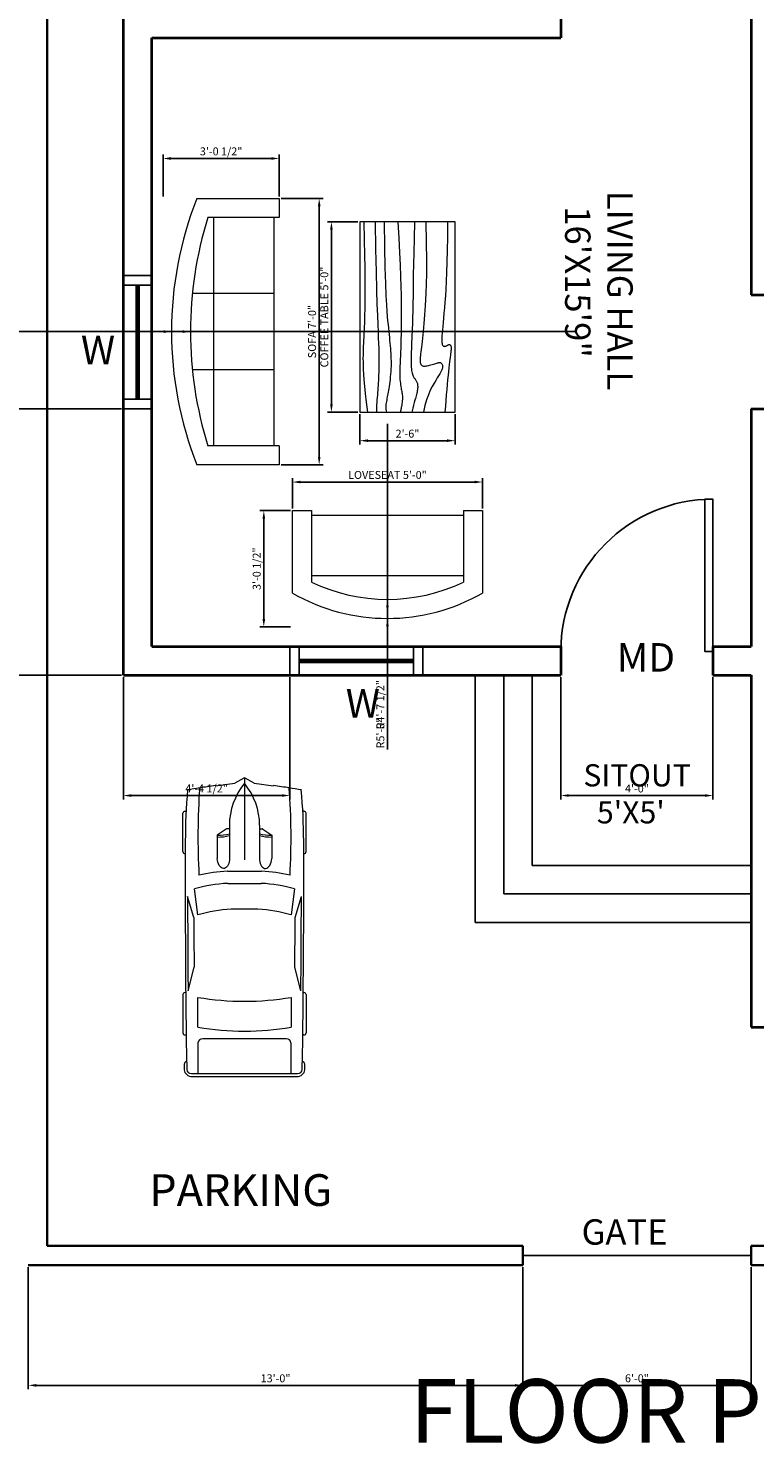
# Model space of a CAD drawing. Units: inches. Extents: x 6038 to 7543, y 3772 to 5131.
# Tile 5 of 14: x 6291 to 6521, y 4306 to 4753. Entities that reach past the tile are written whole.
import ezdxf

# ---------------------------------------------------------------- set-up
doc = ezdxf.new("R2010")
doc.units = ezdxf.units.IN
for name, color, linetype, lineweight in [('A-ANNO-DIMS', 4, 'Continuous', 18), ('A-ANNO-TEXT', 7, 'Continuous', 18), ('A-ANNO-TITL', 3, 'Continuous', 30), ('A-AREA-IDEN', 2, 'Continuous', 18), ('A-DOOR', 3, 'Continuous', 25), ('A-FLOR-STRS', 7, 'Continuous', 25), ('A-FURN', 8, 'Continuous', 18), ('A-SITE-VEHC', 8, 'Continuous', 18), ('A-WALL', 7, 'Continuous', 40)]:
    doc.layers.add(name, color=color, linetype=linetype, lineweight=lineweight)
doc.layers.add('A-GLAZ', color=30, linetype='Continuous', lineweight=25, true_color=0xf26722)
doc.layers.add('C-PROP-WALL', color=251, linetype='Continuous', lineweight=35, true_color=0x636466)
doc.styles.get("Standard").update_dxf_attribs({"font": 'arial.ttf'})
doc.dimstyles.new('ISO-25', dxfattribs={"dimtxt": 2.5, "dimasz": 2.5, "dimexe": 1.25, "dimexo": 0.625, "dimtad": 1, "dimdec": 0, "dimlunit": 3, "dimtxsty": 'Standard', "dimcen": 2.5, "dimadec": 0, "dimazin": 0, "dimtfac": 1, "dimtdec": 0, "dimtmove": 0, "dimatfit": 3, "dimfxl": 1, "dimarcsym": 0})

# ---------------------------------------------------------------- blocks, each defined once
blk = doc.blocks.new('Sofa - Roundback 7 ft.')
for p, q in [((-12.00002, -32.4421), (-12.00003, -6.5971)), ((11.99997, -32.4421), (11.99998, -6.5971)), ((-36.000027, -34), (-36.000027, -11.4696)), ((-35.999844, -13.3819), (35.9998, -13.3819)), ((35.99998, -34), (35.99998, -11.4696)), ((-36.000027, -32.4421), (35.99998, -32.4421))]:
    blk.add_line(p, q)
for points in [[(-36.000027, -34), (-42.000027, -34), (-42.000027, -8)], [(41.99998, -8), (41.99998, -34), (35.99998, -34)]]:
    blk.add_lwpolyline(points)
for centre, radius, start, end in [((0, -114.25), 114.25, 68.43141, 111.5686), ((-0.00001, -127.1968), 121.1968, 72.72033, 107.2797)]:
    blk.add_arc(centre, radius, start, end)
blk = doc.blocks.new('Sofa - Roundback Loveseat 5 ft.')
for p, q in [((0, -32.44198), (0, -5.99998)), ((-24, -33.99998), (-24, -11.46958)), ((-23.9998, -13.38178), (23.99986, -13.38178)), ((24.00004, -33.99998), (24.00004, -11.46958)), ((-24, -32.44198), (24.00004, -32.44198))]:
    blk.add_line(p, q)
for points in [[(-24, -33.99998), (-30, -33.99998), (-30, -7.99998)], [(30.00004, -7.99998), (30.00004, -33.99998), (24.00004, -33.99998)]]:
    blk.add_lwpolyline(points)
for centre, radius, start, end in [((0, -60.24998), 60.24998, 60.13715, 119.8628), ((0, -61.38438), 55.38444, 64.32083, 115.6792)]:
    blk.add_arc(centre, radius, start, end)
blk = doc.blocks.new('Table - Rectangular Woodgrain 60 x 30 in.')
for p, q in [((0, 0), (0, -30)), ((60, 0), (0, 0)), ((60, -30), (60, 0)), ((0, -30), (60, -30))]:
    blk.add_line(p, q)
for points in [[(0, -2.4), (4.8155, -2.418), (9.0302, -2.4688), (12.709, -2.5477), (15.9167, -2.65), (18.7181, -2.7711), (21.1781, -2.9063), (23.3616, -3.0508), (25.3333, -3.2), (27.1477, -3.3495), (28.8172, -3.4958), (30.3437, -3.636), (31.7291, -3.7667), (32.9756, -3.8849), (34.0849, -3.9875), (35.059, -4.0714), (35.9, -4.1334), (36.6114, -4.1711), (37.2041, -4.1854), (37.6906, -4.1779), (38.0833, -4.15), (38.3948, -4.1034), (38.6375, -4.0396), (38.8239, -3.9602), (38.9666, -3.8667), (39.0764, -3.7608), (39.1573, -3.6448), (39.2116, -3.521), (39.2416, -3.3917), (39.2498, -3.2593), (39.2385, -3.1261), (39.21, -2.9944), (39.1666, -2.8667), (39.111, -2.7447), (39.0468, -2.6281), (38.978, -2.5163), (38.9083, -2.4083), (38.8418, -2.3035), (38.7823, -2.201), (38.7337, -2.1001), (38.7, -2), (38.6844, -1.9003), (38.6875, -1.8021), (38.7094, -1.707), (38.75, -1.6167), (38.8094, -1.5326), (38.8875, -1.4563), (38.9844, -1.3893), (39.1, -1.3333), (39.2351, -1.2896), (39.3937, -1.2583), (39.5804, -1.2396), (39.8, -1.2333), (40.057, -1.2396), (40.3562, -1.2583), (40.7023, -1.2896), (41.1, -1.3333), (41.5547, -1.3895), (42.0755, -1.4573), (42.6721, -1.5361), (43.3542, -1.625), (44.1316, -1.7233), (45.014, -1.8302), (46.0114, -1.9449), (47.1333, -2.0667), (48.3862, -2.1947), (49.7625, -2.3281), (51.2513, -2.4663), (52.8416, -2.6083), (54.5226, -2.7535), (56.2833, -2.9011), (58.1127, -3.0501), (60, -3.2)], [(0, -9.2), (6.5759, -9.0858), (11.9385, -9.0365), (16.2527, -9.0418), (19.6833, -9.0917), (22.3952, -9.1759), (24.5531, -9.2844), (26.322, -9.4069), (27.8666, -9.5333), (29.3241, -9.6553), (30.7203, -9.7719), (32.0532, -9.8837), (33.3208, -9.9917), (34.5213, -10.0965), (35.6526, -10.199), (36.7128, -10.2999), (37.7, -10.4), (38.6129, -10.4996), (39.4531, -10.5969), (40.223, -10.6895), (40.925, -10.775), (41.5613, -10.8512), (42.1344, -10.9156), (42.6465, -10.966), (43.1, -11), (43.4976, -11.0158), (43.8437, -11.0136), (44.143, -10.9942), (44.4, -10.9583), (44.6195, -10.9069), (44.8062, -10.8406), (44.9648, -10.7603), (45.1, -10.6667), (45.2155, -10.5598), (45.3114, -10.4365), (45.3871, -10.2929), (45.4416, -10.125), (45.4743, -9.929), (45.4844, -9.7011), (45.4709, -9.4371), (45.4333, -9.1333), (45.3716, -8.7883), (45.2896, -8.4104), (45.1919, -8.0107), (45.0833, -7.6), (44.9685, -7.1893), (44.8521, -6.7896), (44.7388, -6.4117), (44.6333, -6.0667), (44.54, -5.7628), (44.4614, -5.4979), (44.4001, -5.2675), (44.3583, -5.0667), (44.3384, -4.8909), (44.3427, -4.7354), (44.3736, -4.5956), (44.4333, -4.4667), (44.5236, -4.3453), (44.6427, -4.2333), (44.7884, -4.1339), (44.9583, -4.05), (45.1501, -3.9849), (45.3614, -3.9417), (45.59, -3.9234), (45.8333, -3.9333), (46.0915, -3.9749), (46.3734, -4.0531), (46.6906, -4.1736), (47.0542, -4.3417), (47.4756, -4.5629), (47.9661, -4.8427), (48.5372, -5.1866), (49.2, -5.6), (49.9676, -6.0844), (50.8594, -6.625), (51.8965, -7.2031), (53.1, -7.8), (54.491, -8.3969), (56.0906, -8.975), (57.9199, -9.5156), (60, -10)], [(0, -12.8), (5.1847, -12.9322), (9.6213, -13.0323), (13.3963, -13.1059), (16.5958, -13.1583), (19.3063, -13.1952), (21.614, -13.2219), (23.6054, -13.2439), (25.3666, -13.2667), (26.9728, -13.2947), (28.4531, -13.3281), (29.8256, -13.3663), (31.1083, -13.4083), (32.3191, -13.4535), (33.476, -13.501), (34.597, -13.5501), (35.7, -13.6), (36.7984, -13.6497), (37.8875, -13.6979), (38.9578, -13.743), (40, -13.7833), (41.0047, -13.8174), (41.9625, -13.8438), (42.864, -13.8607), (43.7, -13.8667), (44.4631, -13.8604), (45.1552, -13.8417), (45.7801, -13.8104), (46.3416, -13.7667), (46.8439, -13.7104), (47.2906, -13.6417), (47.6858, -13.5604), (48.0333, -13.4667), (48.3375, -13.3608), (48.6042, -13.2448), (48.8396, -13.121), (49.05, -12.9917), (49.2417, -12.8593), (49.4208, -12.7261), (49.5937, -12.5944), (49.7667, -12.4667), (49.9452, -12.3451), (50.1323, -12.2313), (50.3303, -12.1268), (50.5416, -12.0333), (50.7686, -11.9524), (51.0135, -11.8854), (51.2788, -11.8341), (51.5666, -11.8), (51.8785, -11.7843), (52.2116, -11.7865), (52.562, -11.8059), (52.926, -11.8417), (53.2998, -11.8931), (53.6795, -11.9594), (54.0614, -12.0397), (54.4416, -12.1333), (54.8223, -12.2401), (55.2293, -12.3625), (55.6942, -12.5037), (56.2489, -12.6667), (56.9251, -12.8547), (57.7545, -13.0708), (58.7689, -13.3182), (60, -13.6)], [(0, -18), (5.124, -17.7273), (9.6609, -17.5057), (13.6705, -17.3303), (17.2125, -17.1958), (20.3467, -17.0973), (23.1328, -17.0297), (25.6307, -16.9878), (27.9, -16.9667), (29.9928, -16.9617), (31.9302, -16.9703), (33.7254, -16.9907), (35.3917, -17.0208), (36.9423, -17.0588), (38.3906, -17.1026), (39.7499, -17.1503), (41.0333, -17.2), (42.2519, -17.2496), (43.4073, -17.2969), (44.4986, -17.3395), (45.525, -17.375), (46.4858, -17.4012), (47.3802, -17.4156), (48.2074, -17.416), (48.9667, -17.4), (49.6583, -17.3662), (50.2872, -17.3167), (50.8595, -17.2547), (51.3812, -17.1833), (51.8584, -17.1057), (52.2971, -17.025), (52.7034, -16.9443), (53.0833, -16.8667), (53.443, -16.7951), (53.789, -16.7313), (54.128, -16.6768), (54.4666, -16.6334), (54.8115, -16.6024), (55.1693, -16.5854), (55.5465, -16.5841), (55.95, -16.6), (56.3828, -16.6337), (56.8346, -16.6823), (57.2915, -16.7418), (57.7396, -16.8084), (58.165, -16.878), (58.5539, -16.9469), (58.8924, -17.0111), (59.1666, -17.0667), (59.3679, -17.1107), (59.5078, -17.1438), (59.6032, -17.1675), (59.6708, -17.1833), (59.7275, -17.193), (59.7901, -17.1979), (59.8753, -17.1998), (60, -17.2)], [(0, -22.4), (8.0098, -22.2501), (14.4094, -22.1011), (19.4168, -21.9535), (23.25, -21.8083), (26.1269, -21.6663), (28.2656, -21.5281), (29.884, -21.3947), (31.2, -21.2667), (32.3967, -21.1448), (33.5172, -21.0292), (34.5697, -20.9198), (35.5625, -20.8167), (36.5037, -20.7198), (37.4015, -20.6292), (38.2642, -20.5448), (39.1, -20.4667), (39.9164, -20.3951), (40.7187, -20.3313), (41.5117, -20.2768), (42.3, -20.2333), (43.0883, -20.2024), (43.8812, -20.1854), (44.6836, -20.1841), (45.5, -20.2), (46.3328, -20.234), (47.1747, -20.2844), (48.0163, -20.3488), (48.8479, -20.425), (49.66, -20.5106), (50.4429, -20.6031), (51.1872, -20.7004), (51.8833, -20.8), (52.5246, -20.8999), (53.1166, -20.9995), (53.6681, -21.0983), (54.1875, -21.1958), (54.6834, -21.2919), (55.1646, -21.3859), (55.6394, -21.4777), (56.1167, -21.5667), (56.6028, -21.6515), (57.0961, -21.7266), (57.5929, -21.7852), (58.0896, -21.8208), (58.5823, -21.8268), (59.0674, -21.7964), (59.5412, -21.723), (60, -21.6)], [(0, -25.2), (8.6355, -25.0504), (15.7026, -24.9031), (21.4049, -24.7606), (25.9458, -24.625), (29.529, -24.4988), (32.3578, -24.3844), (34.6359, -24.284), (36.5667, -24.2), (38.3213, -24.1341), (39.9417, -24.0854), (41.437, -24.0523), (42.8167, -24.0333), (44.0901, -24.0268), (45.2667, -24.0313), (46.3557, -24.0451), (47.3667, -24.0667), (48.309, -24.0947), (49.1928, -24.1287), (50.0284, -24.168), (50.826, -24.2125), (51.5959, -24.2617), (52.3483, -24.3151), (53.0935, -24.3725), (53.8417, -24.4334), (54.6009, -24.497), (55.3699, -24.561), (56.1454, -24.6226), (56.9239, -24.6792), (57.7021, -24.7279), (58.4764, -24.7662), (59.2435, -24.7911), (60, -24.8)], [(0, -28.8), (5.6867, -28.6681), (10.45, -28.5698), (14.407, -28.5012), (17.675, -28.4584), (20.3711, -28.4374), (22.6125, -28.4344), (24.5164, -28.4455), (26.2, -28.4667), (27.762, -28.4947), (29.2276, -28.5281), (30.6033, -28.5663), (31.8958, -28.6084), (33.1118, -28.6535), (34.2578, -28.7011), (35.3405, -28.7501), (36.3666, -28.8), (37.3443, -28.8497), (38.288, -28.8974), (39.2137, -28.9412), (40.1375, -28.9792), (41.0753, -29.0093), (42.0432, -29.0297), (43.0572, -29.0384), (44.1333, -29.0333), (45.2936, -29.0114), (46.5843, -28.9641), (48.0579, -28.8816), (49.7666, -28.7542), (51.7629, -28.5721), (54.0989, -28.3255), (56.8272, -28.0048), (60, -27.6)]]:
    blk.add_lwpolyline(points)
blk = doc.blocks.new('*U9')
for p, q in [((0, 0), (0, -6)), ((36, 0), (36, -6))]:
    blk.add_line(p, q)
blk.add_lwpolyline([(0, 0), (0, 36), (1.75, 36), (1.75, 0)], close=True)
blk.add_arc((0, 0), 36, 0, 90)
blk = doc.blocks.new('*U10')
for p, q in [((-32, 0), (-32, -5)), ((0, 0), (0, -5))]:
    blk.add_line(p, q)
blk.add_lwpolyline([(0, 0), (0, 32), (-1.75, 32), (-1.75, 0)], close=True)
blk.add_arc((0, 0), 32, 90, 180)
blk = doc.blocks.new('*U12')
for p, q in [((536, 950), (536, 936)), ((1182, 988), (568, 988)), ((1214, 950), (1214, 950)), ((2235, 810), (1899, 912)), ((3440, 942), (3440, 950)), ((3472, 988), (4087, 988)), ((4119, 950), (4119, 934)), ((1779, 801), (2195, 746)), ((3412, 904), (3030, 807)), ((3516, 746), (3994, 746)), ((4736, 746), (4242, 746)), ((4736, -851), (4736, 851)), ((4785, -832), (4785, 832)), ((4179, 670), (4179, -670)), ((756, 241), (1313, 241)), ((816, 241), (816, 283)), ((820, 295), (918, 436)), ((918, 436), (1294, 436)), ((1496, -274), (1496, 274)), ((1690, -267), (1690, 267)), ((4736, -267), (4736, 267)), ((83, 156), (3, 10)), ((2102, 216), (2102, -216)), ((0, 0), (1313, 0)), ((3, -10), (83, -156)), ((756, -241), (1313, -241)), ((816, -241), (816, -283)), ((820, -295), (918, -436)), ((918, -436), (1294, -436)), ((2195, -746), (1779, -801)), ((2235, -810), (1899, -912)), ((3412, -904), (3030, -807)), ((3994, -746), (3516, -746)), ((4242, -746), (4736, -746)), ((536, -950), (536, -936)), ((1182, -988), (568, -988)), ((1214, -950), (1214, -950)), ((3440, -942), (3440, -950)), ((3472, -988), (4087, -988)), ((4119, -950), (4119, -934))]:
    blk.add_line(p, q)
for centre, major_axis, ratio, start_param, end_param in [((6757, -699), (0, 7958), 0.842304, 1.367076, 1.39176), ((1046, -12468), (0, 13417), 0.842304, 0.00281, 0.075598), ((568, 950), (0, -37.6), 0.842304, 3.141593, 4.712389), ((1638, -268113), (0, 269063), 0.842304, -0.013397, 0.002797), ((1182, 950), (0, 37.6), 0.842304, -1.570796, 0), ((1638, -268113), (0, -269025), 0.842304, 3.133765, 3.140441), ((3472, 950), (0, -37.6), 0.842304, 3.141593, 4.712389), ((4087, 950), (0, 37.6), 0.842304, -1.570796, 0), ((4588, 910), (0, 56.4), 0.842304, -0.013017, 1.249894), ((1638, -268131), (0, 269121), 0.842304, -0.013397, -0.013017), ((4673, 851), (0, -75.2), 0.842304, 1.570796, 3.128196), ((4673, 832), (0, -133), 0.842304, 1.570796, 3.128196), ((6583, -699), (0, -7755), 0.842304, 4.528606, 4.561838), ((952, -15087), (0, -15833), 0.842304, 3.096046, 3.200911), ((3414, 137), (0, -2280), 0.842304, 4.449482, 4.652344), ((3436, 137), (0, 2077), 0.842304, 1.245306, 1.50788), ((3800, 71), (0, -2021), 0.842304, 4.372215, 4.640744), ((2433, -93125), (0, -93935), 0.842304, 3.134049, 3.144098), ((434, 0), (0, 3734), 0.842304, 4.511394, 4.913384), ((912, 0), (0, 3734), 0.842304, 4.511394, 4.913384), ((4242, 670), (0, 75.2), 0.842304, 0, 1.570796), ((-5194, 1331), (0, -6374), 0.842304, 1.385369, 1.434372), ((756, -1185), (0, 1427), 0.842304, 0, 0.590319), ((832, 283), (0, 18.8), 0.842304, 0.879714, 1.570796), ((331, 432), (0, 696), 0.842304, 4.435146, 4.718221), ((361, 432), (0, 696), 0.842304, 4.435146, 4.718221), ((1290, 339), (161, -9), 0.603834, -1.395552, 1.581315), ((16, 0), (0, -18.8), 0.842304, 4.131459, 5.293319), ((-5194, -1331), (0, 6374), 0.842304, -1.434372, -1.385369), ((756, 1185), (0, 1427), 0.842304, 2.551274, 3.141593), ((3800, -71), (0, -2021), 0.842304, -1.499151, -1.230623), ((832, -283), (0, -18.8), 0.842304, 4.712389, 5.403472), ((331, -432), (0, -696), 0.842304, 1.564964, 1.848039), ((361, -432), (0, -696), 0.842304, 1.564964, 1.848039), ((3414, -137), (0, -2280), 0.842304, -1.510751, -1.307889), ((3436, -137), (0, -2077), 0.842304, -1.50788, -1.245306), ((6583, 699), (0, 7755), 0.842304, 1.721348, 1.754579), ((4242, -670), (0, -75.2), 0.842304, 4.712389, 6.283185), ((6757, 699), (0, 7958), 0.842304, 1.749832, 1.774517), ((952, 15087), (0, -15833), 0.842304, -0.059319, 0.045547), ((1638, 268113), (0, -269025), 0.842304, 0.001152, 0.007828), ((2433, 93125), (0, -93935), 0.842304, -0.002505, 0.007544), ((4673, -851), (0, 75.2), 0.842304, 3.15499, 4.712389), ((4673, -832), (0, -133), 0.842304, 0.013397, 1.570796), ((1046, 12468), (0, -13417), 0.842304, -0.075598, -0.00281), ((568, -950), (0, 37.6), 0.842304, 1.570796, 3.141593), ((1638, 268113), (0, 269063), 0.842304, 3.138796, 3.15499), ((1182, -950), (0, -37.6), 0.842304, 0, 1.570796), ((3472, -950), (0, -37.6), 0.842304, -1.570796, 0), ((4087, -950), (0, 37.6), 0.842304, 3.141593, 4.712389), ((4588, -910), (0, -56.4), 0.842304, -1.249894, 0.013017), ((1638, 268131), (0, 269121), 0.842304, 3.15461, 3.15499)]:
    blk.add_ellipse(centre, major_axis=major_axis, ratio=ratio, start_param=start_param, end_param=end_param)
at = {"extrusion": (0, 0, -1)}
blk.add_ellipse((1290, -339), major_axis=(161, 9), ratio=0.603834, start_param=-1.395552, end_param=1.581315, dxfattribs=at)
blk = doc.blocks.new('*D15')
at = {"layer": 'A-ANNO-DIMS', "color": 0, "lineweight": -2, "transparency": 16777216}
for p, q in [((6320.79, 4893.62), (6264.12, 4893.62)), ((6265.37, 4891.12), (6265.37, 4551.12)), ((6320.79, 4548.62), (6264.12, 4548.62))]:
    blk.add_line(p, q, dxfattribs=at)
at = {"layer": 'A-ANNO-DIMS', "color": 0, "transparency": 16777216}
for points in [[(6264.96, 4891.12), (6265.79, 4891.12), (6265.37, 4893.62)], [(6264.96, 4551.12), (6265.79, 4551.12), (6265.37, 4548.62)]]:
    blk.add_solid(points, dxfattribs=at)
at = {"layer": 'Defpoints', "color": 0, "transparency": 16777216}
for p in [(6321.42, 4893.62), (6265.37, 4548.62), (6321.42, 4548.62)]:
    blk.add_point(p, dxfattribs=at)
at = {"layer": 'A-ANNO-DIMS', "color": 0, "transparency": 16777216, "insert": (6257.09, 4721.12), "char_height": 2.5, "attachment_point": 5, "rotation": 90}
blk.add_mtext('{\\H6x;28\'-9"}', dxfattribs=at)
blk = doc.blocks.new('WIN-36-PLAN')
for p, q in [((9, 42), (0, 42)), ((9, 39), (0, 39)), ((4, 39), (4, 3)), ((4.5, 39), (4.5, 3)), ((5, 39), (5, 3)), ((9, 3), (0, 3)), ((9, 0), (0, 0))]:
    blk.add_line(p, q)
blk = doc.blocks.new('*D38')
at = {"layer": 'A-ANNO-DIMS', "color": 0, "lineweight": -2, "transparency": 16777216}
for p, q in [((6371.22, 4698.97), (6384.44, 4698.97)), ((6383.19, 4617.47), (6383.19, 4696.47)), ((6371.22, 4614.97), (6384.44, 4614.97))]:
    blk.add_line(p, q, dxfattribs=at)
at = {"layer": 'A-ANNO-DIMS', "color": 0, "transparency": 16777216}
for points in [[(6382.77, 4696.47), (6383.61, 4696.47), (6383.19, 4698.97)], [(6382.77, 4617.47), (6383.61, 4617.47), (6383.19, 4614.97)]]:
    blk.add_solid(points, dxfattribs=at)
at = {"layer": 'Defpoints', "color": 0, "transparency": 16777216}
for p in [(6370.59, 4698.97), (6383.19, 4698.97), (6370.59, 4614.97)]:
    blk.add_point(p, dxfattribs=at)
at = {"layer": 'A-ANNO-DIMS', "color": 0, "transparency": 16777216, "insert": (6381.27, 4656.97), "char_height": 2.5, "attachment_point": 5, "rotation": 90}
blk.add_mtext('SOFA 7\'-0"', dxfattribs=at)
blk = doc.blocks.new('*D39')
at = {"layer": 'A-ANNO-DIMS', "color": 0, "lineweight": -2, "transparency": 16777216}
for p, q in [((6333.92, 4699.6), (6333.92, 4712.82)), ((6368.09, 4711.57), (6336.42, 4711.57)), ((6370.59, 4699.6), (6370.59, 4712.82))]:
    blk.add_line(p, q, dxfattribs=at)
at = {"layer": 'A-ANNO-DIMS', "color": 0, "transparency": 16777216}
for points in [[(6336.42, 4711.99), (6336.42, 4711.15), (6333.92, 4711.57)], [(6368.09, 4711.99), (6368.09, 4711.15), (6370.59, 4711.57)]]:
    blk.add_solid(points, dxfattribs=at)
at = {"layer": 'Defpoints', "color": 0, "transparency": 16777216}
for p in [(6333.92, 4711.57), (6333.92, 4698.97), (6370.59, 4698.97)]:
    blk.add_point(p, dxfattribs=at)
at = {"layer": 'A-ANNO-DIMS', "color": 0, "transparency": 16777216, "insert": (6352.26, 4713.49), "char_height": 2.5, "attachment_point": 5}
blk.add_mtext('3\'-0 1/2"', dxfattribs=at)
blk = doc.blocks.new('*D40')
at = {"layer": 'A-ANNO-DIMS', "color": 0, "lineweight": -2, "transparency": 16777216}
for p, q in [((6374.72, 4601.16), (6374.72, 4610.78)), ((6434.72, 4601.16), (6434.72, 4610.78)), ((6432.22, 4609.53), (6377.22, 4609.53))]:
    blk.add_line(p, q, dxfattribs=at)
at = {"layer": 'A-ANNO-DIMS', "color": 0, "transparency": 16777216}
for points in [[(6377.22, 4609.95), (6377.22, 4609.12), (6374.72, 4609.53)], [(6432.22, 4609.95), (6432.22, 4609.12), (6434.72, 4609.53)]]:
    blk.add_solid(points, dxfattribs=at)
at = {"layer": 'Defpoints', "color": 0, "transparency": 16777216}
for p in [(6374.72, 4609.53), (6374.72, 4600.53), (6434.72, 4600.53)]:
    blk.add_point(p, dxfattribs=at)
at = {"layer": 'A-ANNO-DIMS', "color": 0, "transparency": 16777216, "insert": (6404.72, 4611.45), "char_height": 2.5, "attachment_point": 5}
blk.add_mtext('LOVESEAT 5\'-0"', dxfattribs=at)
blk = doc.blocks.new('*D41')
at = {"layer": 'A-ANNO-DIMS', "color": 0, "lineweight": -2, "transparency": 16777216}
for p, q in [((6374.1, 4600.53), (6364.47, 4600.53)), ((6365.72, 4598.03), (6365.72, 4566.37)), ((6374.1, 4563.87), (6364.47, 4563.87))]:
    blk.add_line(p, q, dxfattribs=at)
at = {"layer": 'A-ANNO-DIMS', "color": 0, "transparency": 16777216}
for points in [[(6365.3, 4598.03), (6366.14, 4598.03), (6365.72, 4600.53)], [(6365.3, 4566.37), (6366.14, 4566.37), (6365.72, 4563.87)]]:
    blk.add_solid(points, dxfattribs=at)
at = {"layer": 'Defpoints', "color": 0, "transparency": 16777216}
for p in [(6374.72, 4600.53), (6365.72, 4563.87), (6374.72, 4563.87)]:
    blk.add_point(p, dxfattribs=at)
at = {"layer": 'A-ANNO-DIMS', "color": 0, "transparency": 16777216, "insert": (6363.8, 4582.2), "char_height": 2.5, "attachment_point": 5, "rotation": 90}
blk.add_mtext('3\'-0 1/2"', dxfattribs=at)
blk = doc.blocks.new('*D42')
at = {"layer": 'A-ANNO-DIMS', "color": 0, "lineweight": -2, "transparency": 16777216}
for p, q in [((6395.42, 4691.57), (6385.79, 4691.57)), ((6387.04, 4689.07), (6387.04, 4634.07)), ((6395.42, 4631.57), (6385.79, 4631.57))]:
    blk.add_line(p, q, dxfattribs=at)
at = {"layer": 'A-ANNO-DIMS', "color": 0, "transparency": 16777216}
for points in [[(6386.63, 4689.07), (6387.46, 4689.07), (6387.04, 4691.57)], [(6386.63, 4634.07), (6387.46, 4634.07), (6387.04, 4631.57)]]:
    blk.add_solid(points, dxfattribs=at)
at = {"layer": 'Defpoints', "color": 0, "transparency": 16777216}
for p in [(6396.04, 4691.57), (6387.04, 4631.57), (6396.04, 4631.57)]:
    blk.add_point(p, dxfattribs=at)
at = {"layer": 'A-ANNO-DIMS', "color": 0, "transparency": 16777216, "insert": (6385.13, 4661.57), "char_height": 2.5, "attachment_point": 5, "rotation": 90}
blk.add_mtext('COFFEE TABLE 5\'-0"', dxfattribs=at)
blk = doc.blocks.new('*D43')
at = {"layer": 'A-ANNO-DIMS', "color": 0, "lineweight": -2, "transparency": 16777216}
for p, q in [((6396.04, 4630.95), (6396.04, 4621.32)), ((6426.04, 4630.95), (6426.04, 4621.32)), ((6398.54, 4622.57), (6423.54, 4622.57))]:
    blk.add_line(p, q, dxfattribs=at)
at = {"layer": 'A-ANNO-DIMS', "color": 0, "transparency": 16777216}
for points in [[(6398.54, 4622.99), (6398.54, 4622.16), (6396.04, 4622.57)], [(6423.54, 4622.99), (6423.54, 4622.16), (6426.04, 4622.57)]]:
    blk.add_solid(points, dxfattribs=at)
at = {"layer": 'Defpoints', "color": 0, "transparency": 16777216}
for p in [(6396.04, 4631.57), (6426.04, 4631.57), (6426.04, 4622.57)]:
    blk.add_point(p, dxfattribs=at)
at = {"layer": 'A-ANNO-DIMS', "color": 0, "transparency": 16777216, "insert": (6411.04, 4624.47), "char_height": 2.5, "attachment_point": 5}
blk.add_mtext('2\'-6"', dxfattribs=at)
blk = doc.blocks.new('*D52')
at = {"layer": 'A-ANNO-DIMS', "color": 0, "lineweight": -2, "transparency": 16777216}
for p, q in [((6291.42, 4361.99), (6291.42, 4323.42)), ((6447.42, 4361.99), (6447.42, 4323.42)), ((6293.92, 4324.67), (6444.92, 4324.67))]:
    blk.add_line(p, q, dxfattribs=at)
at = {"layer": 'A-ANNO-DIMS', "color": 0, "transparency": 16777216}
for points in [[(6293.92, 4325.09), (6293.92, 4324.25), (6291.42, 4324.67)], [(6444.92, 4325.09), (6444.92, 4324.25), (6447.42, 4324.67)]]:
    blk.add_solid(points, dxfattribs=at)
at = {"layer": 'Defpoints', "color": 0, "transparency": 16777216}
for p in [(6291.42, 4362.62), (6447.42, 4362.62), (6447.42, 4324.67)]:
    blk.add_point(p, dxfattribs=at)
at = {"layer": 'A-ANNO-DIMS', "color": 0, "transparency": 16777216, "insert": (6369.42, 4326.57), "char_height": 2.5, "attachment_point": 5}
blk.add_mtext('13\'-0"', dxfattribs=at)
blk = doc.blocks.new('*D53')
at = {"layer": 'A-ANNO-DIMS', "color": 0, "lineweight": -2, "transparency": 16777216}
for p, q in [((6447.42, 4361.99), (6447.42, 4323.42)), ((6519.42, 4361.99), (6519.42, 4323.42)), ((6449.92, 4324.67), (6516.92, 4324.67))]:
    blk.add_line(p, q, dxfattribs=at)
at = {"layer": 'A-ANNO-DIMS', "color": 0, "transparency": 16777216}
for points in [[(6449.92, 4325.09), (6449.92, 4324.25), (6447.42, 4324.67)], [(6516.92, 4325.09), (6516.92, 4324.25), (6519.42, 4324.67)]]:
    blk.add_solid(points, dxfattribs=at)
at = {"layer": 'Defpoints', "color": 0, "transparency": 16777216}
for p in [(6447.42, 4362.62), (6519.42, 4362.62), (6519.42, 4324.67)]:
    blk.add_point(p, dxfattribs=at)
at = {"layer": 'A-ANNO-DIMS', "color": 0, "transparency": 16777216, "insert": (6483.42, 4326.57), "char_height": 2.5, "attachment_point": 5}
blk.add_mtext('6\'-0"', dxfattribs=at)
blk = doc.blocks.new('*D57')
at = {"layer": 'A-ANNO-DIMS', "color": 0, "lineweight": -2, "transparency": 16777216}
for p, q in [((6459.42, 4547.99), (6459.42, 4509.42)), ((6507.42, 4547.99), (6507.42, 4509.42)), ((6504.92, 4510.67), (6461.92, 4510.67))]:
    blk.add_line(p, q, dxfattribs=at)
at = {"layer": 'A-ANNO-DIMS', "color": 0, "transparency": 16777216}
for points in [[(6461.92, 4511.09), (6461.92, 4510.25), (6459.42, 4510.67)], [(6504.92, 4511.09), (6504.92, 4510.25), (6507.42, 4510.67)]]:
    blk.add_solid(points, dxfattribs=at)
at = {"layer": 'Defpoints', "color": 0, "transparency": 16777216}
for p in [(6459.42, 4548.62), (6507.42, 4548.62), (6459.42, 4510.67)]:
    blk.add_point(p, dxfattribs=at)
at = {"layer": 'A-ANNO-DIMS', "color": 0, "transparency": 16777216, "insert": (6483.42, 4512.57), "char_height": 2.5, "attachment_point": 5}
blk.add_mtext('4\'-0"', dxfattribs=at)
blk = doc.blocks.new('*D63')
at = {"layer": 'A-ANNO-DIMS', "color": 0, "lineweight": -2, "transparency": 16777216}
for p, q in [((6320.79, 4632.62), (6252.22, 4632.62)), ((6253.47, 4551.12), (6253.47, 4630.12)), ((6320.79, 4548.62), (6252.22, 4548.62))]:
    blk.add_line(p, q, dxfattribs=at)
at = {"layer": 'A-ANNO-DIMS', "color": 0, "transparency": 16777216}
for points in [[(6253.05, 4630.12), (6253.88, 4630.12), (6253.47, 4632.62)], [(6253.05, 4551.12), (6253.88, 4551.12), (6253.47, 4548.62)]]:
    blk.add_solid(points, dxfattribs=at)
at = {"layer": 'Defpoints', "color": 0, "transparency": 16777216}
for p in [(6253.47, 4632.62), (6321.42, 4632.62), (6321.42, 4548.62)]:
    blk.add_point(p, dxfattribs=at)
at = {"layer": 'A-ANNO-DIMS', "color": 0, "transparency": 16777216, "insert": (6251.57, 4590.62), "char_height": 2.5, "attachment_point": 5, "rotation": 90}
blk.add_mtext('7\'-0"', dxfattribs=at)
blk = doc.blocks.new('*D64')
at = {"layer": 'A-ANNO-DIMS', "color": 0, "lineweight": -2, "transparency": 16777216}
for p, q in [((6321.42, 4547.99), (6321.42, 4509.42)), ((6373.92, 4547.99), (6373.92, 4509.42)), ((6371.42, 4510.67), (6323.92, 4510.67))]:
    blk.add_line(p, q, dxfattribs=at)
at = {"layer": 'A-ANNO-DIMS', "color": 0, "transparency": 16777216}
for points in [[(6323.92, 4511.09), (6323.92, 4510.25), (6321.42, 4510.67)], [(6371.42, 4511.09), (6371.42, 4510.25), (6373.92, 4510.67)]]:
    blk.add_solid(points, dxfattribs=at)
at = {"layer": 'Defpoints', "color": 0, "transparency": 16777216}
for p in [(6321.42, 4548.62), (6373.92, 4548.62), (6321.42, 4510.67)]:
    blk.add_point(p, dxfattribs=at)
at = {"layer": 'A-ANNO-DIMS', "color": 0, "transparency": 16777216, "insert": (6347.67, 4512.59), "char_height": 2.5, "attachment_point": 5}
blk.add_mtext('4\'-4 1/2"', dxfattribs=at)
blk = doc.blocks.new('*D94')
at = {"layer": 'A-ANNO-DIMS', "color": 0, "lineweight": -2, "transparency": 16777216}
for p, q in [((6263.76, 4656.97), (6340.09, 4656.97)), ((6463.79, 4656.97), (6342.59, 4656.97))]:
    blk.add_line(p, q, dxfattribs=at)
at = {"layer": 'A-ANNO-DIMS', "color": 0, "transparency": 16777216}
blk.add_solid([(6340.09, 4657.39), (6340.09, 4656.55), (6342.59, 4656.97)], dxfattribs=at)
at = {"layer": 'Defpoints', "color": 0, "transparency": 16777216}
for p in [(6342.59, 4656.97), (6463.79, 4656.97)]:
    blk.add_point(p, dxfattribs=at)
at = {"layer": 'A-ANNO-DIMS', "color": 0, "transparency": 16777216, "insert": (6269.87, 4658.87), "char_height": 2.5, "attachment_point": 5, "rotation": 0.0002}
blk.add_mtext('R10\'-1"', dxfattribs=at)
blk = doc.blocks.new('*D95')
at = {"layer": 'A-ANNO-DIMS', "color": 0, "lineweight": -2, "transparency": 16777216}
for p, q in [((6259.98, 4656.97), (6334.09, 4656.97)), ((6450.84, 4656.97), (6336.59, 4656.97))]:
    blk.add_line(p, q, dxfattribs=at)
at = {"layer": 'A-ANNO-DIMS', "color": 0, "transparency": 16777216}
blk.add_solid([(6334.09, 4657.39), (6334.09, 4656.55), (6336.59, 4656.97)], dxfattribs=at)
at = {"layer": 'Defpoints', "color": 0, "transparency": 16777216}
for p in [(6336.59, 4656.97), (6450.84, 4656.97)]:
    blk.add_point(p, dxfattribs=at)
at = {"layer": 'A-ANNO-DIMS', "color": 0, "transparency": 16777216, "insert": (6268.04, 4658.89), "char_height": 2.5, "attachment_point": 5, "rotation": 0.0002}
blk.add_mtext('R9\'-6 1/2"', dxfattribs=at)
blk = doc.blocks.new('*D96')
at = {"layer": 'A-ANNO-DIMS', "color": 0, "lineweight": -2, "transparency": 16777216}
for p, q in [((6404.72, 4626.78), (6404.72, 4566.53)), ((6404.72, 4525.24), (6404.72, 4564.03))]:
    blk.add_line(p, q, dxfattribs=at)
at = {"layer": 'A-ANNO-DIMS', "color": 0, "transparency": 16777216}
blk.add_solid([(6404.3, 4564.03), (6405.14, 4564.03), (6404.72, 4566.53)], dxfattribs=at)
at = {"layer": 'Defpoints', "color": 0, "transparency": 16777216}
for p in [(6404.72, 4626.78), (6404.72, 4566.53)]:
    blk.add_point(p, dxfattribs=at)
at = {"layer": 'A-ANNO-DIMS', "color": 0, "transparency": 16777216, "insert": (6402.82, 4530.38), "char_height": 2.5, "attachment_point": 5, "rotation": 89.9996}
blk.add_mtext('R5\'-0"', dxfattribs=at)
blk = doc.blocks.new('*D97')
at = {"layer": 'A-ANNO-DIMS', "color": 0, "lineweight": -2, "transparency": 16777216}
for p, q in [((6404.72, 4627.92), (6404.72, 4572.53)), ((6404.72, 4531.25), (6404.72, 4570.03))]:
    blk.add_line(p, q, dxfattribs=at)
at = {"layer": 'A-ANNO-DIMS', "color": 0, "transparency": 16777216}
blk.add_solid([(6404.3, 4570.03), (6405.14, 4570.03), (6404.72, 4572.53)], dxfattribs=at)
at = {"layer": 'Defpoints', "color": 0, "transparency": 16777216}
for p in [(6404.72, 4627.92), (6404.72, 4572.53)]:
    blk.add_point(p, dxfattribs=at)
at = {"layer": 'A-ANNO-DIMS', "color": 0, "transparency": 16777216, "insert": (6402.8, 4539.3), "char_height": 2.5, "attachment_point": 5, "rotation": 89.9996}
blk.add_mtext('R4\'-7 1/2"', dxfattribs=at)

msp = doc.modelspace()

# ---------------------------------------------------------------- linework, layer by layer
at = {"layer": 'A-DOOR'}
msp.add_line((6447.42, 4365.62), (6519.42, 4365.62), dxfattribs=at)
at = {"layer": 'A-FLOR-STRS'}
for p, q in [((6432.42, 4548.62), (6432.42, 4470.62)), ((6441.42, 4548.62), (6441.42, 4479.62)), ((6450.42, 4548.62), (6450.42, 4488.62)), ((6450.42, 4488.62), (6519.42, 4488.62)), ((6441.42, 4479.62), (6519.42, 4479.62)), ((6432.42, 4470.62), (6519.42, 4470.62))]:
    msp.add_line(p, q, dxfattribs=at)
at = {"layer": 'A-WALL'}
for p, q in [((6321.42, 4548.62), (6321.42, 4956.62)), ((6519.42, 4773.62), (6519.42, 4668.62)), ((6459.42, 4755.62), (6459.42, 4749.62)), ((6330.42, 4749.62), (6459.42, 4749.62)), ((6330.42, 4557.62), (6330.42, 4749.62)), ((6519.42, 4668.62), (6528.42, 4668.62)), ((6519.42, 4632.62), (6528.42, 4632.62)), ((6519.42, 4632.62), (6519.42, 4557.62)), ((6330.42, 4557.62), (6459.42, 4557.62)), ((6459.42, 4557.62), (6459.42, 4548.62)), ((6507.42, 4557.62), (6507.42, 4548.62)), ((6507.42, 4557.62), (6519.42, 4557.62)), ((6321.42, 4548.62), (6459.42, 4548.62)), ((6507.42, 4548.62), (6519.42, 4548.62)), ((6519.42, 4548.62), (6519.42, 4437.62)), ((6519.42, 4437.62), (6672.42, 4437.62))]:
    msp.add_line(p, q, dxfattribs=at)
at = {"layer": 'C-PROP-WALL'}
for p, q in [((6297.42, 4368.62), (6297.42, 4980.62)), ((6330.42, 4368.62), (6297.42, 4368.62)), ((6447.42, 4368.62), (6330.42, 4368.62)), ((6447.42, 4368.62), (6447.42, 4362.62)), ((6672.42, 4368.62), (6519.42, 4368.62)), ((6519.42, 4368.62), (6519.42, 4362.62)), ((6447.42, 4362.62), (6291.42, 4362.62)), ((6711.42, 4362.62), (6519.42, 4362.62))]:
    msp.add_line(p, q, dxfattribs=at)

# ---------------------------------------------------------------- block references
at = {"layer": 'A-DOOR', "rotation": 270}
msp.add_blockref('*U9', (6525.42, 4668.62), dxfattribs=at)
at = {"layer": 'A-DOOR', "xscale": 1.5, "yscale": 1.5, "zscale": 1.5}
msp.add_blockref('*U10', (6507.42, 4556.12), dxfattribs=at)
at = {"layer": 'A-FURN'}
for name, p, rotation in [('Sofa - Roundback 7 ft.', (6336.59, 4656.97), 90), ('Table - Rectangular Woodgrain 60 x 30 in.', (6426.04, 4691.57), 270), ('Sofa - Roundback Loveseat 5 ft.', (6404.72, 4566.53), 180)]:
    msp.add_blockref(name, p, dxfattribs=dict(at, rotation=rotation))
at = {"layer": 'A-GLAZ'}
msp.add_blockref('WIN-36-PLAN', (6321.42, 4632.62), dxfattribs=at)
at = {"layer": 'A-GLAZ', "rotation": 89.9999999999961}
msp.add_blockref('WIN-36-PLAN', (6415.92, 4548.62), dxfattribs=at)
at = {"layer": 'A-SITE-VEHC', "xscale": 0.0196850393700788, "yscale": 0.0196850393700788, "zscale": 0.0196850393700788, "rotation": 270}
msp.add_blockref('*U12', (6359.62, 4516.24), dxfattribs=at)

# ---------------------------------------------------------------- texts
at = {"layer": 'A-ANNO-TEXT', "attachment_point": 1}
for s, width, insert, char_height in [('W', 212.1416, (6308.02, 4655.65), 9), ('MD', 212.1416, (6477.04, 4558.74), 9), ('W', 212.1416, (6391.58, 4544.23), 9), ('GATE', 365.6257, (6465.96, 4377.04), 8)]:
    msp.add_mtext_dynamic_manual_height_columns(s, width=width, gutter_width=12.5, heights=[0], dxfattribs=dict(at, insert=insert, char_height=char_height))
at = {"layer": 'A-ANNO-TITL', "insert": (6411.79, 4326.63), "char_height": 20, "attachment_point": 1}
msp.add_mtext_dynamic_manual_height_columns('FLOOR PLAN', width=549.9641, gutter_width=12.5, heights=[0], dxfattribs=at)
at = {"layer": 'A-AREA-IDEN', "insert": (6482.1, 4701.39), "char_height": 8, "attachment_point": 1, "rotation": 270}
msp.add_mtext_dynamic_manual_height_columns('LIVING HALL\\P  16\'X15\'9"', width=1254.8618, gutter_width=12.5, heights=[0], dxfattribs=at)
at = {"layer": 'A-AREA-IDEN', "attachment_point": 1}
for s, width, insert, char_height in [("SITOUT\\P  5'X5'", 295.3899, (6466.53, 4520.55), 7), ('PARKING', 447.2968, (6329.58, 4391.26), 10)]:
    msp.add_mtext_dynamic_manual_height_columns(s, width=width, gutter_width=12.5, heights=[0], dxfattribs=dict(at, insert=insert, char_height=char_height))

# ---------------------------------------------------------------- dimensions: what is measured, and where the dimension line sits
at = {"layer": 'A-ANNO-DIMS'}
for base, p1, p2, angle, text, override, picture, middle in [((6265.37, 4548.62), (6321.42, 4893.62), (6321.42, 4548.62), 90, '{\\H6x;<>}', {"dimclrd": 0, "dimclre": 0, "dimclrt": 0}, '*D15', (6257.09, 4721.12)), ((6383.19, 4698.97), (6370.59, 4614.97), (6370.59, 4698.97), 90, 'SOFA <>', {"dimdec": 1, "dimlfac": 1, "dimrnd": 0, "dimzin": 1, "dimdsep": 46, "dimlunit": 4, "dimfrac": 2}, '*D38', (6381.27, 4656.97)), ((6387.04, 4631.57), (6396.04, 4691.57), (6396.04, 4631.57), 270, 'COFFEE TABLE <>', {"dimdec": 1, "dimlfac": 1, "dimrnd": 0, "dimzin": 1, "dimdsep": 46, "dimlunit": 4, "dimfrac": 2}, '*D42', (6385.13, 4661.57)), ((6374.72, 4609.53), (6434.72, 4600.53), (6374.72, 4600.53), 180, 'LOVESEAT <>', {"dimdec": 1, "dimlfac": 1, "dimrnd": 0, "dimzin": 1, "dimdsep": 46, "dimlunit": 4, "dimfrac": 2}, '*D40', (6404.72, 4611.45))]:
    dim = msp.add_linear_dim(base=base, p1=p1, p2=p2, angle=angle, text=text, dimstyle='ISO-25', override=override, dxfattribs=at)
    dim.commit()
    dim.dimension.update_dxf_attribs({"geometry": picture, "text_midpoint": middle})
for base, p1, p2, angle, picture, middle in [((6333.92, 4711.57), (6370.59, 4698.97), (6333.92, 4698.97), 180, '*D39', (6352.26, 4713.49)), ((6253.47, 4632.62), (6321.42, 4548.62), (6321.42, 4632.62), 90, '*D63', (6251.57, 4590.62)), ((6365.72, 4563.87), (6374.72, 4600.53), (6374.72, 4563.87), 270, '*D41', (6363.8, 4582.2)), ((6321.42, 4510.67), (6373.92, 4548.62), (6321.42, 4548.62), 180, '*D64', (6347.67, 4512.59)), ((6459.42, 4510.67), (6507.42, 4548.62), (6459.42, 4548.62), 180, '*D57', (6483.42, 4512.57))]:
    dim = msp.add_linear_dim(base=base, p1=p1, p2=p2, angle=angle, dimstyle='ISO-25', override={"dimdec": 1, "dimlfac": 1, "dimrnd": 0, "dimzin": 1, "dimdsep": 46, "dimlunit": 4, "dimfrac": 2}, dxfattribs=at)
    dim.commit()
    dim.dimension.update_dxf_attribs({"geometry": picture, "text_midpoint": middle})
for center, mpoint, picture, middle in [((6450.840765, 4656.970422), (6336.590765, 4656.97), '*D95', (6268.040765, 4656.9697468)), ((6463.79, 4656.97), (6342.59, 4656.97), '*D94', (6269.87, 4656.97)), ((6404.72, 4627.92), (6404.72, 4572.53), '*D97', (6404.72, 4539.3)), ((6404.72041, 4626.78378), (6404.72, 4566.5338), '*D96', (6404.71976, 4530.38382))]:
    dim = msp.add_radius_dim(center=center, mpoint=mpoint, dimstyle='ISO-25', override={"dimdec": 1, "dimlfac": 1, "dimrnd": 0, "dimzin": 1, "dimdsep": 46, "dimlunit": 4, "dimfrac": 2}, dxfattribs=at)
    dim.commit()
    dim.dimension.update_dxf_attribs({"geometry": picture, "text_midpoint": middle, "dimtype": 164})
for base, p1, p2, picture, middle in [((6426.04, 4622.57), (6396.04, 4631.57), (6426.04, 4631.57), '*D43', (6411.04, 4624.47)), ((6447.42, 4324.67), (6291.42, 4362.62), (6447.42, 4362.62), '*D52', (6369.42, 4326.57)), ((6519.42, 4324.67), (6447.42, 4362.62), (6519.42, 4362.62), '*D53', (6483.42, 4326.57))]:
    dim = msp.add_linear_dim(base=base, p1=p1, p2=p2, dimstyle='ISO-25', override={"dimdec": 1, "dimlfac": 1, "dimrnd": 0, "dimzin": 1, "dimdsep": 46, "dimlunit": 4, "dimfrac": 2}, dxfattribs=at)
    dim.commit()
    dim.dimension.update_dxf_attribs({"geometry": picture, "text_midpoint": middle})

doc.saveas('drawing.dxf')
